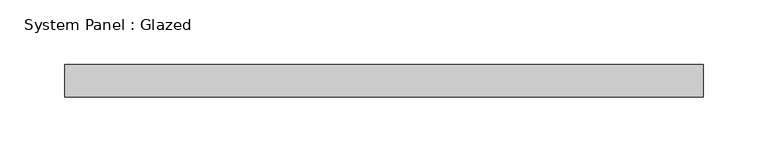
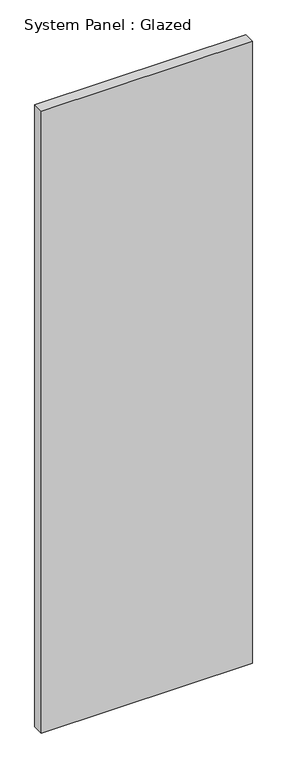
"""IFC4 building model written with IfcOpenShell, lengths in millimetres: plate geometry, System Panel : Glazed."""

from ifc_helpers import new_model, si_unit, origin, origin_with_axes, place, context, project, spatial, polyline, outline, extrude, source, transform, mapped, element, save


def system_panel_glazed_0fd7ce52(model_context):
    return source(origin(), model_context, "Body", "SweptSolid", [
        extrude(outline(polyline([(247.65, 19.05), (-247.65, 19.05), (-247.65, 44.45), (247.65, 44.45), (247.65, 19.05)])), origin_with_axes(), (0.0, 0.0, 1.0), 1540.45282),
    ])


if __name__ == "__main__":
    model = new_model("IFC4")
    model_context = context("Model", 3, world=origin())
    ifc_project = project(units=[si_unit("LENGTHUNIT", "METRE", prefix="MILLI")], contexts=[model_context])
    site = spatial("IfcSite", under=ifc_project)
    building = spatial("IfcBuilding", under=site)
    placement = place(None, origin())
    system_panel_glazed_shape = system_panel_glazed_0fd7ce52(model_context)
    element("IfcPlate", 1, ObjectType="System Panel : Glazed", at=placement, inside=building, context=model_context, shape_type="MappedRepresentation", body=[
        mapped(system_panel_glazed_shape, transform((0.0, 0.0, 0.0), x_axis=(1.0, 0.0, 0.0), y_axis=(0.0, 1.0, 0.0), z_axis=(0.0, 0.0, 1.0))),
    ])
    save(model, "model.ifc")

# Revit data of these elements
# Type "System Panel : Glazed"
#   Construction Type Id = "GSP4R"
#   Analytic Construction = "1/8 in Pilkington single glazing"
#   Visual Light Transmittance = 0.9
#   Solar Heat Gain Coefficient = 0.86
#   Heat Transfer Coefficient (U) = 1.18115 BTU/(h·ft²·°F)
#   Define Thermal Properties by = 1
# Element 1 (IfcPlate, "System Panel : Glazed")
#   Materials on its faces: "Glass"
# Materials
#   "Glass": class "Glass", colour RGB 0 128 192, transparency 0.75, Description = "Soda Lime Glass", Cost = 0
